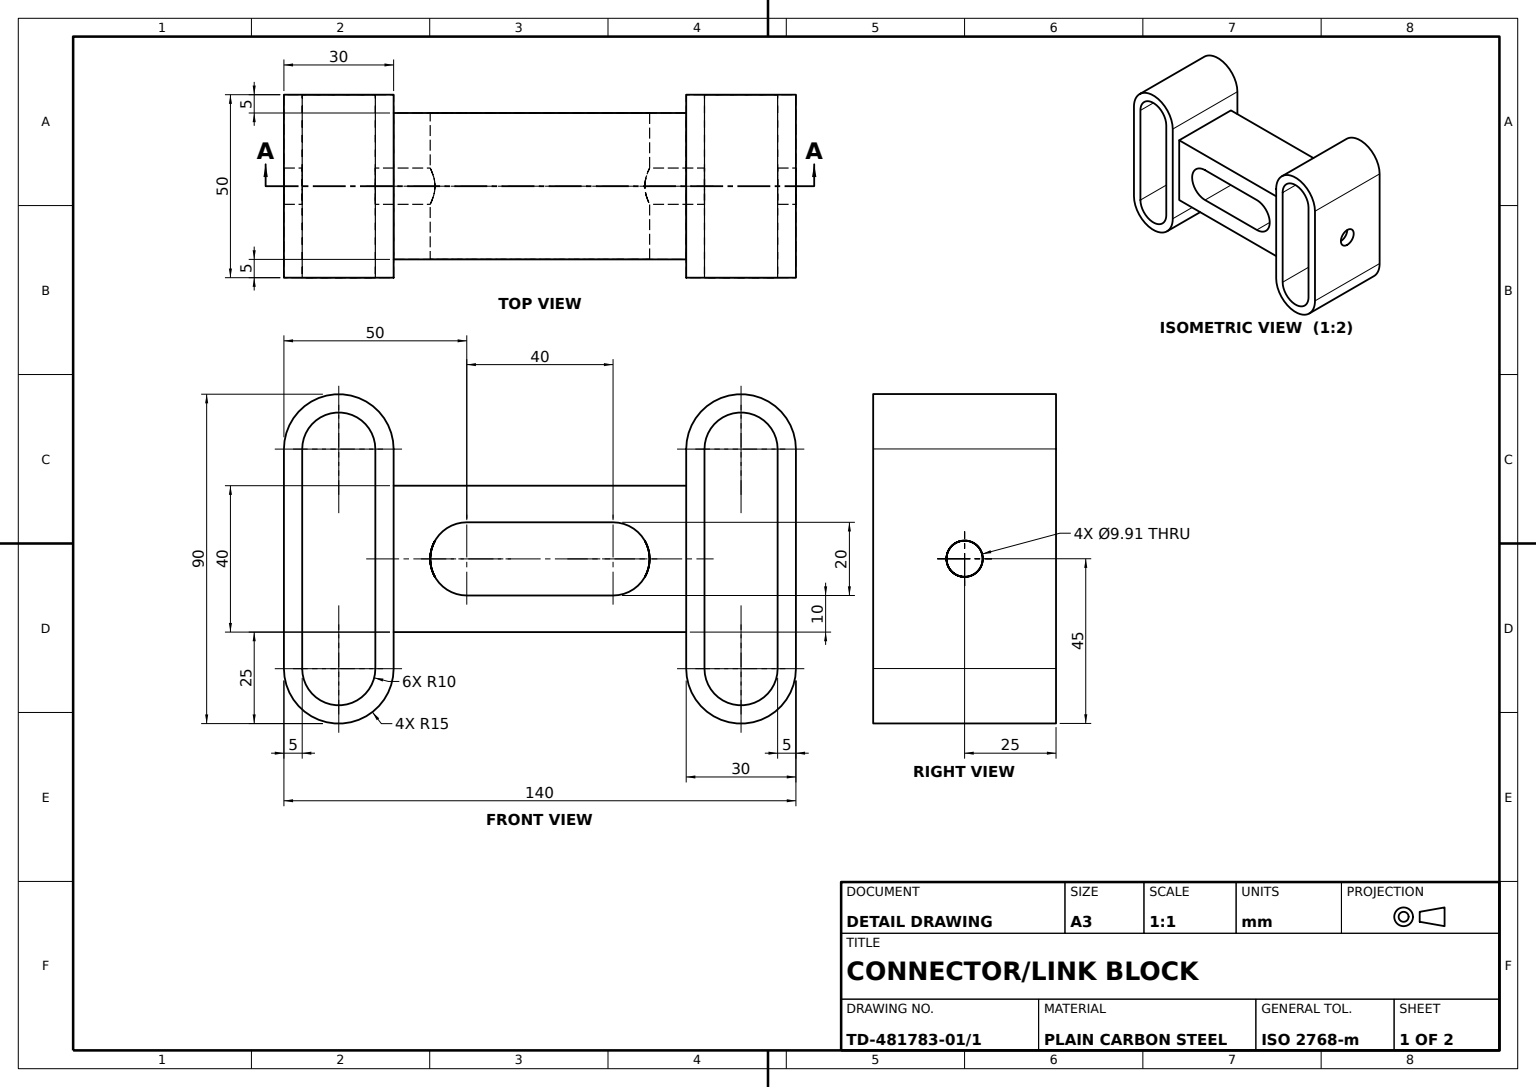
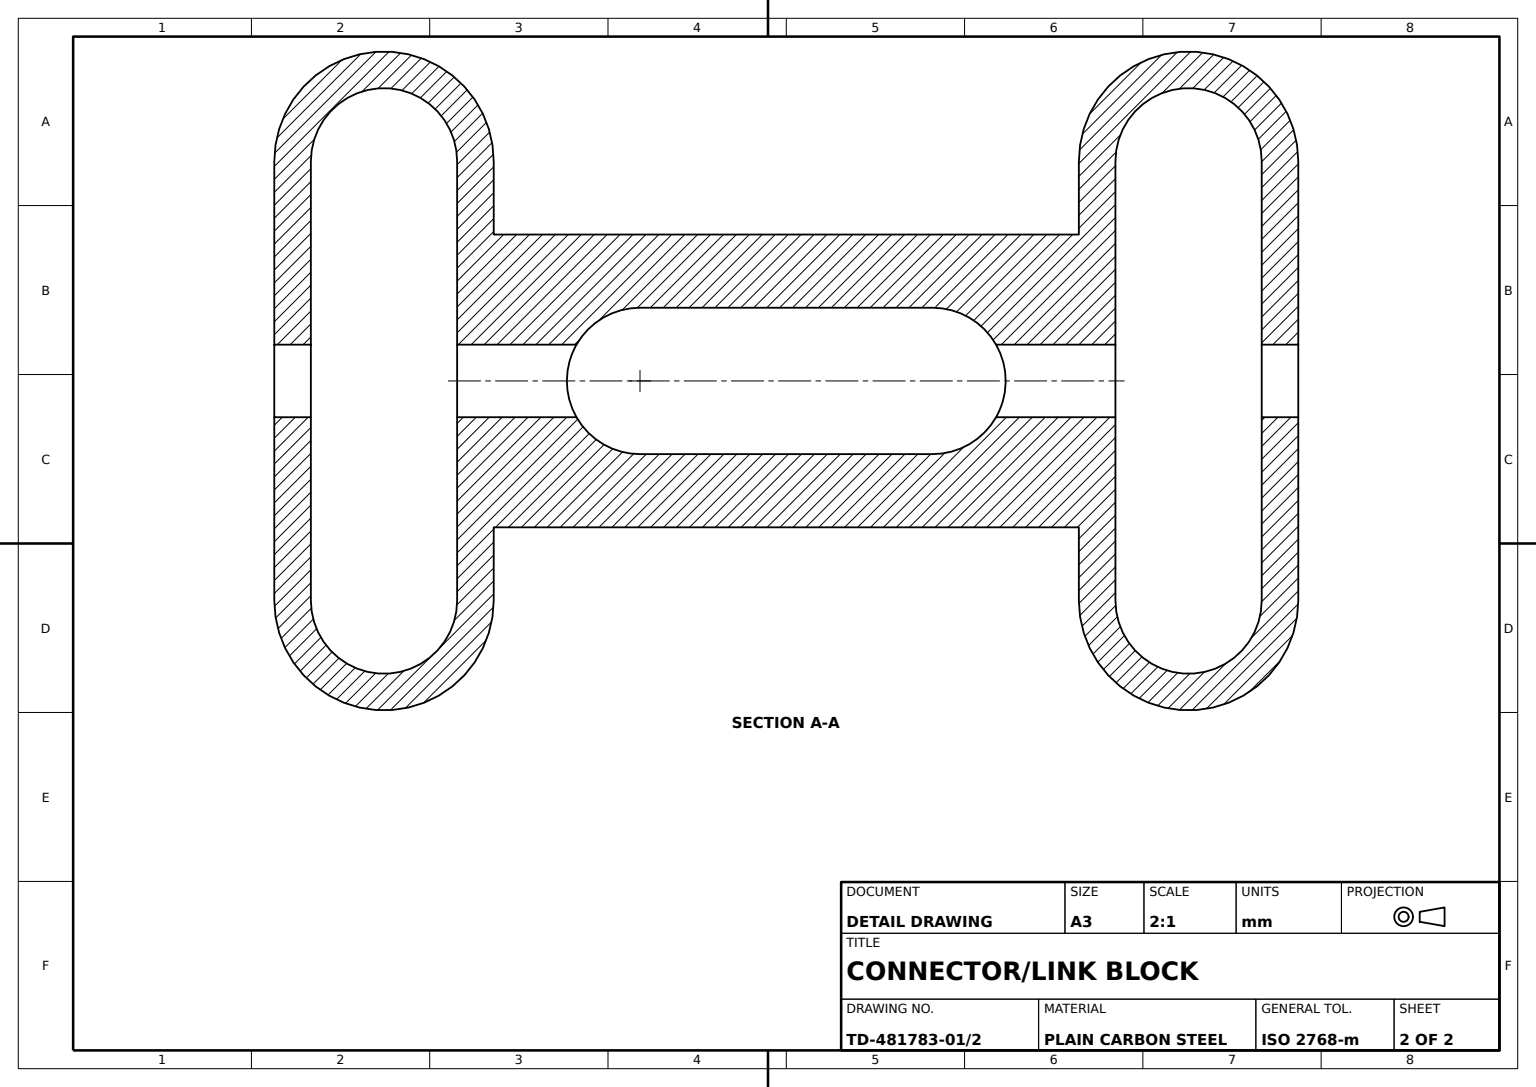
SolidWorks part; units mm, degrees
material "Plain Carbon Steel"
ref_plane "Front Plane" through (0, 0, 0) normal (0, 0, 1) x (1, 0, 0)
ref_plane "Top Plane" through (0, 0, 0) normal (0, 1, 0) x (1, 0, 0)
ref_plane "Right Plane" through (0, 0, 0) normal (1, 0, 0) x (0, 0, -1)
sketch "End Loops Sketch" plane through (0, 0, 0) normal (0, 0, 1) x (1, 0, 0)
  line L0 (-40, 5) -> (65, 5)
  line L1 (55, 35) -> (55, -25) construction
  line L4 (-55, 35) -> (-55, -25) construction
  line L5 (-45, 35) -> (-45, -25)
  line L6 (-65, 35) -> (-65, -25)
  line L7 (-55, 35) -> (-55, -25) construction
  line L8 (-40, 35) -> (-40, -25)
  line L9 (-70, 35) -> (-70, -25)
  line L10 (70, 35) -> (70, -25)
  line L11 (40, 35) -> (40, -25)
  line L12 (55, 35) -> (55, -25) construction
  line L13 (65, 35) -> (65, -25)
  line L14 (45, 35) -> (45, -25)
  arc A0 (-45, 35) -> (-65, 35) centre (-55, 35) ccw
  arc A1 (-65, -25) -> (-45, -25) centre (-55, -25) ccw
  arc A2 (-40, 35) -> (-70, 35) centre (-55, 35) ccw
  arc A3 (-70, -25) -> (-40, -25) centre (-55, -25) ccw
  arc A4 (70, 35) -> (40, 35) centre (55, 35) ccw
  arc A5 (40, -25) -> (70, -25) centre (55, -25) ccw
  arc A6 (65, 35) -> (45, 35) centre (55, 35) ccw
  arc A7 (45, -25) -> (65, -25) centre (55, -25) ccw
  point P3 (-55, 50)
  point P4 (0, 0)
  point P7 (55, 5)
  point P9 (-55, -40)
  point P10 (55, 50)
  point P13 (-55, 5)
  point P20 (-55, 5)
  point P30 (55, 5)
  point P35 (55, -40)
  dimension "D4" = 10
  dimension "D5" = 15
  dimension "D2" = 15
  dimension "D6" = 10
  dimension "D1" = 90
  dimension "D3" = 90
  dimension "D7" = 55
  dimension "D8" = 55
  dimension "D9" = 5
extrude "End Loops" add sketch "End Loops Sketch" along normal mid plane 50
sketch "Centre Block Sketch" plane through (0, 0, 0) normal (0, 0, 1) x (1, 0, 0)
  line L0 (-20, 5) -> (20, 5) construction
  line L2 (40, 35) -> (40, -25) construction
  line L3 (-20, 15) -> (20, 15)
  line L4 (-40, 25) -> (40, 25)
  line L5 (-40, 25) -> (-40, -15)
  line L6 (-40, -15) -> (40, -15)
  line L7 (40, 25) -> (40, -15)
  line L8 (-40, 25) -> (40, -15) construction
  line L9 (-40, -15) -> (40, 25) construction
  line L10 (-20, -5) -> (20, -5)
  arc A0 (-20, 15) -> (-20, -5) centre (-20, 5) ccw
  arc A1 (20, -5) -> (20, 15) centre (20, 5) ccw
  point P2 (0, 5)
  point P6 (0, 5)
  dimension "D1" = 40
  dimension "D2" = 20
  dimension "D3" = 40
  dimension "D4" = 5
extrude "Centre Block" add sketch "Centre Block Sketch" along normal mid plane 40
sketch "Cross Hole Sketch" plane through (70, 0, 0) normal (1, 0, 0) x (0, 0, -1)
  line L0 (-25, -40) -> (25, -40) construction
  line L2 (25, 35) -> (25, -25) construction
  circle A0 centre (0, 5) radius 4.9573
  dimension "D2" = 9.9147
  dimension "D1" = 45
  dimension "D3" = 25
extrude "Cross Hole" cut sketch "Cross Hole Sketch" against normal blind 164
